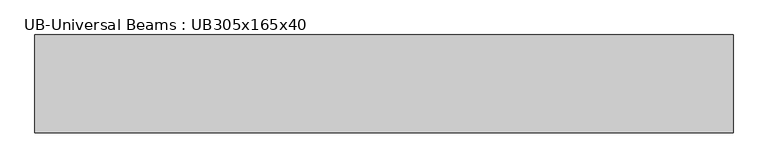
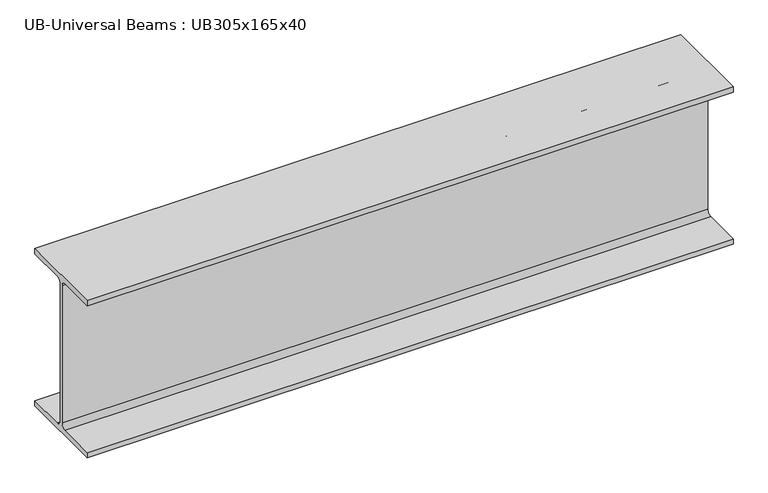
"""IFC4 building model written with IfcOpenShell, lengths in millimetres: beam geometry, UB-Universal Beams : UB305x165x40."""

from ifc_helpers import new_model, si_unit, point, frame, frame_2d, origin, place, context, project, spatial, polyline, circle_curve, trimmed, segment, composite_curve, outline, extrude, source, transform, mapped, element, save


def ub_universal_beams_ub305x165x40_2a071682(model_context):
    return source(origin(), model_context, "Body", "SweptSolid", [
        extrude(outline(composite_curve([segment(polyline([(82.5, -141.5), (82.5, -151.7), (-82.5, -151.7), (-82.5, -141.5), (-11.9, -141.5)]), True, "CONTINUOUS"), segment(trimmed(circle_curve(frame_2d((-11.9, -132.6)), 8.9), [point((-11.9, -141.5))], [point((-3.0, -132.6))], True, "CARTESIAN"), True, "CONTINUOUS"), segment(polyline([(-3.0, -132.6), (-3.0, 132.6)]), True, "CONTINUOUS"), segment(trimmed(circle_curve(frame_2d((-11.9, 132.6)), 8.9), [point((-3.0, 132.6))], [point((-11.9, 141.5))], True, "CARTESIAN"), True, "CONTINUOUS"), segment(polyline([(-11.9, 141.5), (-82.5, 141.5), (-82.5, 151.7), (82.5, 151.7), (82.5, 141.5), (11.9, 141.5)]), True, "CONTINUOUS"), segment(trimmed(circle_curve(frame_2d((11.9, 132.6)), 8.9), [point((11.9, 141.5))], [point((3.0, 132.6))], True, "CARTESIAN"), True, "CONTINUOUS"), segment(polyline([(3.0, 132.6), (3.0, -132.6)]), True, "CONTINUOUS"), segment(trimmed(circle_curve(frame_2d((11.9, -132.6)), 8.9), [point((3.0, -132.6))], [point((11.9, -141.5))], True, "CARTESIAN"), True, "CONTINUOUS"), segment(polyline([(11.9, -141.5), (82.5, -141.5)]), True, "CONTINUOUS")], self_intersect=False)), frame((-789.05, 0.0, 0.0), z_axis=(1.0, 0.0, 0.0), x_axis=(0.0, 1.0, 0.0)), (0.0, 0.0, 1.0), 1176.4),
    ])


if __name__ == "__main__":
    model = new_model("IFC4")
    model_context = context("Model", 3, world=origin())
    ifc_project = project(units=[si_unit("LENGTHUNIT", "METRE", prefix="MILLI")], contexts=[model_context])
    site = spatial("IfcSite", under=ifc_project)
    building = spatial("IfcBuilding", under=site)
    placement = place(None, origin())
    ub_universal_beams_ub305x165x40_shape = ub_universal_beams_ub305x165x40_2a071682(model_context)
    element("IfcBeam", 1, ObjectType="UB-Universal Beams : UB305x165x40", at=placement, inside=building, context=model_context, shape_type="MappedRepresentation", body=[
        mapped(ub_universal_beams_ub305x165x40_shape, transform((0.0, 0.0, 0.0), x_axis=(1.0, 0.0, 0.0), y_axis=(0.0, 1.0, 0.0), z_axis=(0.0, 0.0, 1.0))),
    ])
    save(model, "model.ifc")

# Revit data of these elements
# Type "UB-Universal Beams : UB305x165x40"
#   Section Name Key = "UB305X165X40"
#   Width = 16.5 cm
#   Web Thickness = 0.6 cm
#   Web Fillet = 0.89 cm
#   Warping Constant = 164000.0 cm⁶
#   Torsional Moment of Inertia = 14.70 cm⁴
#   Section Area = 51.3 cm²
#   Plastic Modulus weak axis = 142.0 cm³
#   Plastic Modulus strong axis = 623.0 cm³
#   Nominal Weight = 40.2999 kgf/m
#   Moment of Inertia weak axis = 764.00 cm⁴
#   Moment of Inertia strong axis = 8503.00 cm⁴
#   Height = 30.34 cm
#   Flange Thickness = 1.02 cm
#   Elastic Modulus weak axis = 92.6 cm³
#   Elastic Modulus strong axis = 560.0 cm³
#   Centroid Vertical = 15.17 cm
#   Centroid Horizontal = 8.25 cm
#   Bolt Spacing = 9.0 cm
#   Length [instance default] = 1500 mm
#   Structural Material [instance default] = Metal - Steel 43-275
#   Type Comments = ""
#   Assembly Code = ""
# Element 1 (IfcBeam, "UB-Universal Beams : UB305x165x40")
#   Materials on its faces: "Metal - Steel 43-275"
# Materials
#   "Metal - Steel 43-275": class "Metal", colour RGB 247 247 247, transparency 0, Cost = 0
